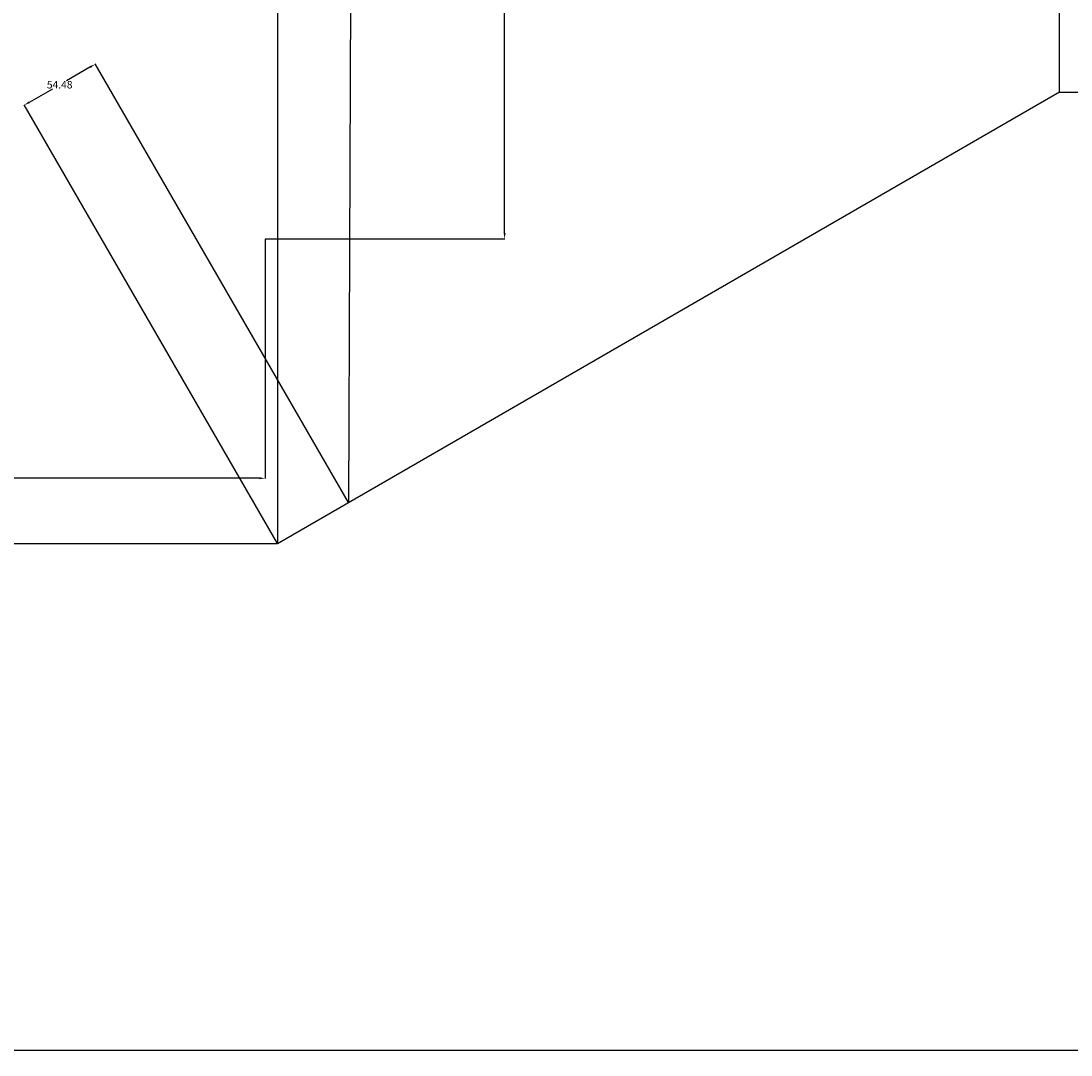
# Model space of a CAD drawing. Units: metres. Extents: x -2391 to 4922, y -635 to 4845.
# Tile 6 of 37: x -659 to 39, y -635 to 53. Entities that reach past the tile are written whole.
import ezdxf

# ---------------------------------------------------------------- set-up
doc = ezdxf.new("R2010")
doc.units = ezdxf.units.M
doc.header["$MEASUREMENT"] = 0
doc.layers.add('A-ANNO-DIMS', color=2, linetype='Continuous', lineweight=18)
doc.layers.add('A-FLOR-FIXT', color=3, linetype='Continuous', lineweight=25)
doc.styles.get("Standard").update_dxf_attribs({"font": 'arial.ttf'})
doc.dimstyles.get("Standard").update_dxf_attribs({"dimtxt": 5, "dimasz": 4, "dimexe": 0.18, "dimexo": 0.0625, "dimgap": 0.09, "dimtad": 0, "dimtih": 1, "dimtoh": 1, "dimdec": 0, "dimzin": 0, "dimdsep": 46, "dimtxsty": 'Standard', "dimcen": 0.09, "dimadec": 0, "dimazin": 0, "dimtfac": 1, "dimtdec": 0, "dimtofl": 0, "dimtmove": 0, "dimatfit": 3, "dimfxl": 1, "dimtolj": 1, "dimtzin": 0, "dimarcsym": 0})

# ---------------------------------------------------------------- blocks, each defined once
blk = doc.blocks.new('*D6')
at = {"layer": 'A-ANNO-DIMS', "color": 0, "lineweight": -2, "transparency": 16777216}
for p, q in [((-496.54, 968.1), (-337.38, 968.1)), ((-337.56, 964.1), (-337.56, 440.64)), ((-337.56, -88.18), (-337.56, 435.28)), ((-496.54, -92.18), (-337.38, -92.18))]:
    blk.add_line(p, q, dxfattribs=at)
at = {"layer": 'A-ANNO-DIMS', "color": 0, "transparency": 16777216}
for points in [[(-338.23, 964.1), (-336.89, 964.1), (-337.56, 968.1)], [(-338.23, -88.18), (-336.89, -88.18), (-337.56, -92.18)]]:
    blk.add_solid(points, dxfattribs=at)
at = {"layer": 'Defpoints', "color": 0, "transparency": 16777216}
for p in [(-496.6, 968.1), (-337.56, 968.1), (-496.6, -92.18)]:
    blk.add_point(p, dxfattribs=at)
at = {"layer": 'A-ANNO-DIMS', "color": 0, "transparency": 16777216, "insert": (-337.56, 437.96), "char_height": 5, "attachment_point": 5}
blk.add_mtext('\\A1;BAR STOOL 1060 TYP.', dxfattribs=at)
blk = doc.blocks.new('*D7')
at = {"layer": 'A-ANNO-DIMS', "color": 0, "lineweight": -2, "transparency": 16777216}
for p, q in [((-1109.41, -92.24), (-1109.41, -251.4)), ((-496.6, -92.24), (-496.6, -251.4)), ((-1105.41, -251.22), (-817.22, -251.22)), ((-500.6, -251.22), (-788.79, -251.22))]:
    blk.add_line(p, q, dxfattribs=at)
at = {"layer": 'A-ANNO-DIMS', "color": 0, "transparency": 16777216}
for points in [[(-1105.41, -250.56), (-1105.41, -251.89), (-1109.41, -251.22)], [(-500.6, -250.56), (-500.6, -251.89), (-496.6, -251.22)]]:
    blk.add_solid(points, dxfattribs=at)
at = {"layer": 'Defpoints', "color": 0, "transparency": 16777216}
for p in [(-1109.41, -92.18), (-496.6, -92.18), (-496.6, -251.22)]:
    blk.add_point(p, dxfattribs=at)
at = {"layer": 'A-ANNO-DIMS', "color": 0, "transparency": 16777216, "insert": (-803, -251.22), "char_height": 5, "attachment_point": 5}
blk.add_mtext('\\A1;613 TYP.', dxfattribs=at)
blk = doc.blocks.new('*D8')
at = {"layer": 'A-ANNO-DIMS', "color": 0, "lineweight": -2, "transparency": 16777216}
for p, q in [((-2047.33, 3005.21), (-2047.33, -631.4)), ((4577.76, 2350.21), (4577.76, -631.4)), ((-2043.33, -631.22), (1257.62, -631.22)), ((4573.76, -631.22), (1272.8, -631.22))]:
    blk.add_line(p, q, dxfattribs=at)
at = {"layer": 'A-ANNO-DIMS', "color": 0, "transparency": 16777216}
for points in [[(-2043.33, -630.56), (-2043.33, -631.89), (-2047.33, -631.22)], [(4573.76, -630.56), (4573.76, -631.89), (4577.76, -631.22)]]:
    blk.add_solid(points, dxfattribs=at)
at = {"layer": 'Defpoints', "color": 0, "transparency": 16777216}
for p in [(-2047.33, 3005.28), (4577.76, 2350.28), (4577.76, -631.22)]:
    blk.add_point(p, dxfattribs=at)
at = {"layer": 'A-ANNO-DIMS', "color": 0, "transparency": 16777216, "insert": (1265.21, -631.22), "char_height": 5, "attachment_point": 5}
blk.add_mtext('\\A1;6625', dxfattribs=at)
blk = doc.blocks.new('*D10')
at = {"layer": 'A-ANNO-DIMS', "color": 0, "lineweight": -2, "transparency": 16777216}
for p, q in [((550.68, 4505.28), (-2384.01, 4505.28)), ((-2383.83, 4501.28), (-2383.83, 2107.92)), ((-2383.83, -290.72), (-2383.83, 2102.63)), ((-488.55, -294.72), (-2384.01, -294.72))]:
    blk.add_line(p, q, dxfattribs=at)
at = {"layer": 'A-ANNO-DIMS', "color": 0, "transparency": 16777216}
for points in [[(-2384.5, 4501.28), (-2383.17, 4501.28), (-2383.83, 4505.28)], [(-2384.5, -290.72), (-2383.17, -290.72), (-2383.83, -294.72)]]:
    blk.add_solid(points, dxfattribs=at)
at = {"layer": 'Defpoints', "color": 0, "transparency": 16777216}
for p in [(-2383.83, 4505.28), (550.74, 4505.28), (-488.49, -294.72)]:
    blk.add_point(p, dxfattribs=at)
at = {"layer": 'A-ANNO-DIMS', "color": 0, "transparency": 16777216, "insert": (-2383.83, 2105.28), "char_height": 5, "attachment_point": 5}
blk.add_mtext('\\A1;4800', dxfattribs=at)
blk = doc.blocks.new('*D48')
at = {"layer": 'A-ANNO-DIMS', "color": 0, "lineweight": -2, "transparency": 16777216}
for p, q in [((31.19, 905.28), (367.81, 905.28)), ((367.63, 901.28), (367.63, 457.92)), ((367.63, 9.28), (367.63, 452.63)), ((31.19, 5.28), (367.81, 5.28))]:
    blk.add_line(p, q, dxfattribs=at)
at = {"layer": 'A-ANNO-DIMS', "color": 0, "transparency": 16777216}
for points in [[(366.96, 901.28), (368.29, 901.28), (367.63, 905.28)], [(366.96, 9.28), (368.29, 9.28), (367.63, 5.28)]]:
    blk.add_solid(points, dxfattribs=at)
at = {"layer": 'Defpoints', "color": 0, "transparency": 16777216}
for p in [(31.13, 905.28), (31.13, 5.28), (367.63, 5.28)]:
    blk.add_point(p, dxfattribs=at)
at = {"layer": 'A-ANNO-DIMS', "color": 0, "transparency": 16777216, "insert": (367.63, 455.28), "char_height": 5, "attachment_point": 5}
blk.add_mtext('\\A1;900', dxfattribs=at)
blk = doc.blocks.new('*D49')
at = {"layer": 'A-ANNO-DIMS', "color": 0, "lineweight": -2, "transparency": 16777216}
for p, q in [((-613.02, 21.93), (-628.57, 12.96)), ((-441.34, -267.43), (-609.65, 24.09)), ((-653.27, -1.31), (-637.73, 7.67)), ((-488.52, -294.67), (-656.83, -3.15))]:
    blk.add_line(p, q, dxfattribs=at)
at = {"layer": 'A-ANNO-DIMS', "color": 0, "transparency": 16777216}
for points in [[(-613.36, 22.51), (-612.69, 21.36), (-609.56, 23.93)], [(-653.61, -0.73), (-652.94, -1.88), (-656.74, -3.31)]]:
    blk.add_solid(points, dxfattribs=at)
at = {"layer": 'Defpoints', "color": 0, "transparency": 16777216}
for p in [(-609.56, 23.93), (-441.31, -267.49), (-488.49, -294.72)]:
    blk.add_point(p, dxfattribs=at)
at = {"layer": 'A-ANNO-DIMS', "color": 0, "transparency": 16777216, "insert": (-633.15, 10.31), "char_height": 5, "attachment_point": 5}
blk.add_mtext('\\A1;54.48', dxfattribs=at)

msp = doc.modelspace()

# ---------------------------------------------------------------- linework, layer by layer
at = {"layer": 'A-FLOR-FIXT'}
for p, q in [((31.1266, 5.2763), (31.1266, 905.2763)), ((-437.841, 634.5176), (-441.31, -267.4852)), ((-488.4886, 605.2763), (-488.4886, -294.7237)), ((31.1266, 5.2763), (-488.4886, -294.7237))]:
    msp.add_line(p, q, dxfattribs=at)

# ---------------------------------------------------------------- dimensions: what is measured, and where the dimension line sits
at = {"layer": 'A-ANNO-DIMS'}
for base, p1, p2, angle, override, picture, middle in [((-2383.8343, 4505.2763), (-488.4886, -294.7237), (550.7419, 4505.2763), 90, {"dimdec": 0, "dimlfac": 1, "dimrnd": 0, "dimzin": 0, "dimdsep": 46, "dimlunit": 2}, '*D10', (-2383.8343, 2105.2763)), ((367.6266, 5.2763), (31.1266, 905.2763), (31.1266, 5.2763), 270, {"dimdec": 0, "dimlfac": 1, "dimrnd": 0, "dimzin": 0, "dimdsep": 46, "dimlunit": 2}, '*D48', (367.6266, 455.2763)), ((-609.56, 23.9324), (-488.4886, -294.7237), (-441.31, -267.4852), 30, {"dimdec": 2, "dimlfac": 1, "dimrnd": 0, "dimzin": 0, "dimdsep": 46, "dimlunit": 2}, '*D49', (-633.1493, 10.3131))]:
    dim = msp.add_linear_dim(base=base, p1=p1, p2=p2, angle=angle, dimstyle='Standard', override=override, dxfattribs=at)
    dim.commit()
    dim.dimension.update_dxf_attribs({"geometry": picture, "text_midpoint": middle})
dim = msp.add_linear_dim(base=(4577.76, -631.2237), p1=(-2047.3343, 3005.2763), p2=(4577.76, 2350.2763), dimstyle='Standard', override={"dimdec": 0, "dimlfac": 1, "dimrnd": 0, "dimzin": 0, "dimdsep": 46, "dimlunit": 2}, dxfattribs=at)
dim.commit()
dim.dimension.update_dxf_attribs({"geometry": '*D8', "text_midpoint": (1265.2128, -631.2237)})
dim = msp.add_linear_dim(base=(-337.5616, 968.1038), p1=(-496.6042, -92.1799), p2=(-496.6042, 968.1038), angle=90, text='BAR STOOL <> TYP.', dimstyle='Standard', override={"dimdec": 0, "dimrnd": 0, "dimzin": 0, "dimlunit": 2}, dxfattribs=at)
dim.commit()
dim.dimension.update_dxf_attribs({"geometry": '*D6', "text_midpoint": (-337.5616, 437.9619)})
dim = msp.add_linear_dim(base=(-496.6042, -251.2224), p1=(-1109.4055, -92.1799), p2=(-496.6042, -92.1799), text='<> TYP.', dimstyle='Standard', override={"dimdec": 0, "dimrnd": 0, "dimzin": 0, "dimlunit": 2}, dxfattribs=at)
dim.commit()
dim.dimension.update_dxf_attribs({"geometry": '*D7', "text_midpoint": (-803.0049, -251.2224)})

doc.saveas('drawing.dxf')
